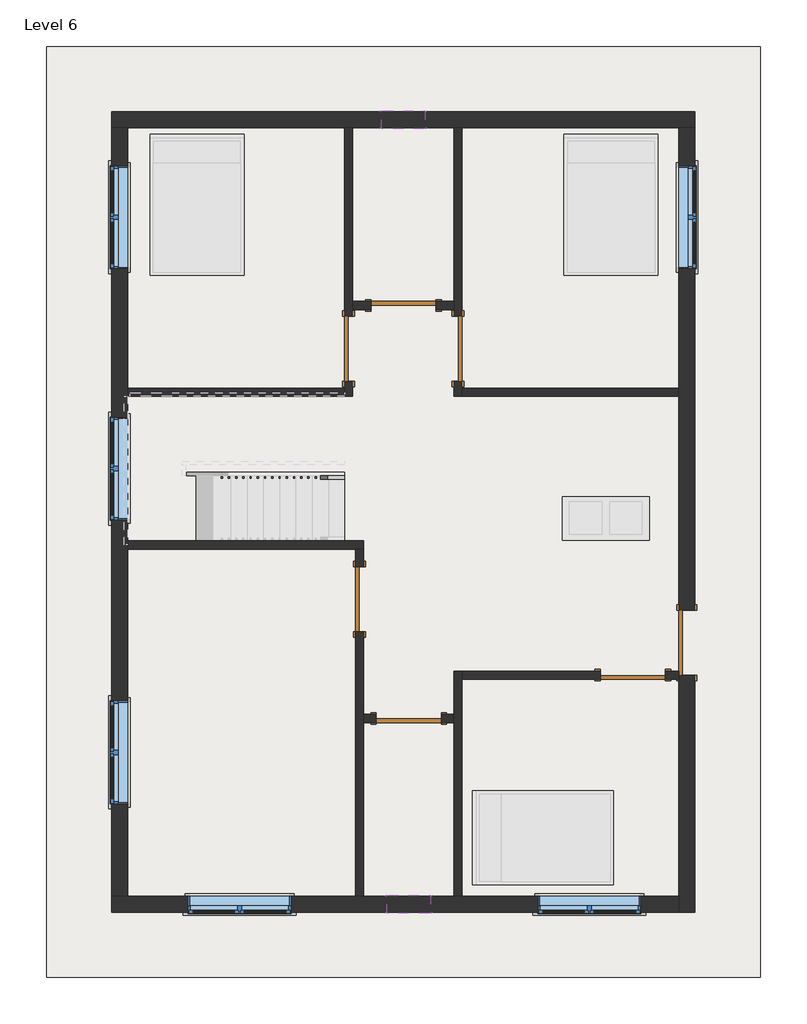
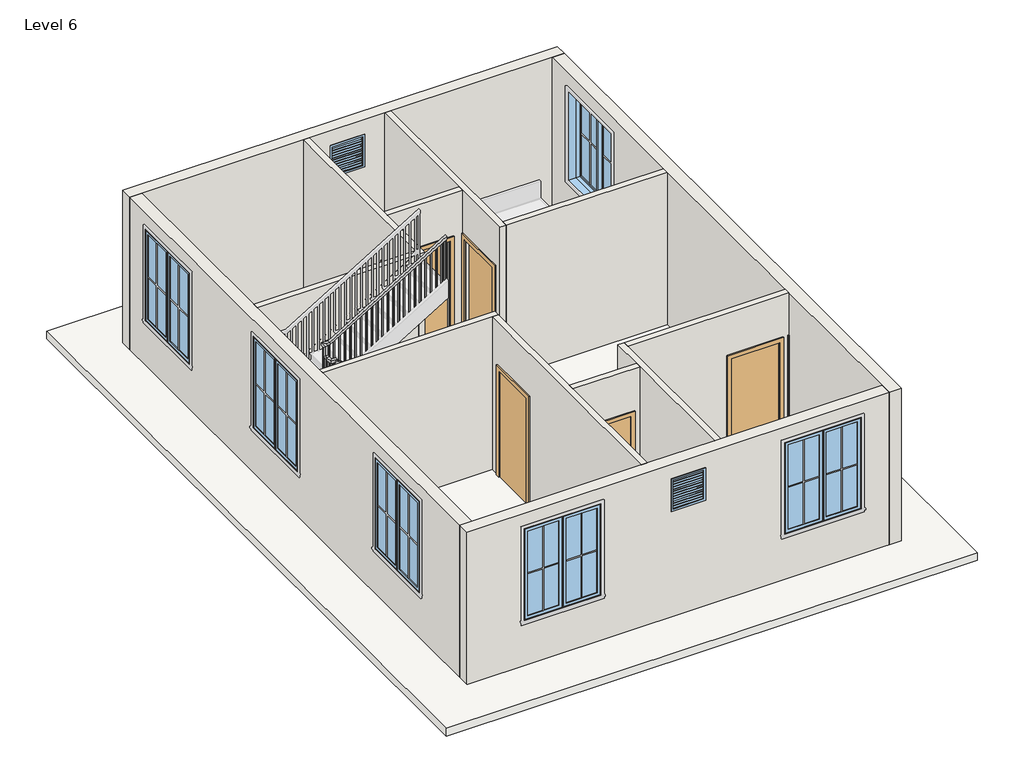
# One storey, part 1 of 2: 14 walls, 8 windows, 7 doors, 1 railing, 1 roof, 1 slab.
"""IFC4 building model written with IfcOpenShell, lengths in millimetres."""

from ifc_helpers import new_model, si_unit, frame, origin, place, context, project, spatial, polyline, outline, extrude, faceted_brep, transform, mapped, element, save
from components import door_305aa2a5, door_e5f9f3c4, door_0ca8825f, window_9ac97e1a, window_f2d8fef0

model = new_model("IFC4")

# Units and contexts
model_context = context("Model", 3, world=origin())
ifc_project = project(units=[si_unit("LENGTHUNIT", "METRE", prefix="MILLI")], contexts=[model_context])

# Site, building, storey
site = spatial("IfcSite", under=ifc_project)
building = spatial("IfcBuilding", under=site)
storey = spatial("IfcBuildingStorey", under=building, Name="Level 6", Elevation=12801.6)

# Doors
placement = place(None, origin())
door_shape = door_305aa2a5(model_context)
element("IfcDoor", 1, ObjectType="Single-Flush : 36\" x 84\"", at=placement, inside=storey, context=model_context, shape_type="MappedRepresentation", body=[
    mapped(door_shape, transform((-2023.6910855, 2116.5303617, 12801.6), x_axis=(0.0, -1.0, 0.0), y_axis=(1.0, 0.0, 0.0), z_axis=(0.0, 0.0, 1.0))),
])
element("IfcDoor", 2, ObjectType="Single-Flush : 36\" x 84\"", at=placement, inside=storey, context=model_context, shape_type="MappedRepresentation", body=[
    mapped(door_shape, transform((-1179.1410855, -3078.1725945, 12801.6), x_axis=(1.0, 0.0, 0.0), y_axis=(0.0, 1.0, 0.0), z_axis=(0.0, 0.0, 1.0))),
])
element("IfcDoor", 3, ObjectType="Single-Flush : 36\" x 84\"", at=placement, inside=storey, context=model_context, shape_type="MappedRepresentation", body=[
    mapped(door_shape, transform((1970.4589145, -2468.1696383, 12801.6), x_axis=(1.0, 0.0, 0.0), y_axis=(0.0, 1.0, 0.0), z_axis=(0.0, 0.0, 1.0))),
])
door_2_shape = door_e5f9f3c4(model_context)
element("IfcDoor", 4, ObjectType="Single-Flush : 36\" x 84\"", at=placement, inside=storey, context=model_context, shape_type="MappedRepresentation", body=[
    mapped(door_2_shape, transform((-486.9910855, 2116.5303617, 12801.6), x_axis=(0.0, -1.0, 0.0), y_axis=(1.0, 0.0, 0.0), z_axis=(0.0, 0.0, 1.0))),
])
element("IfcDoor", 5, ObjectType="Single-Flush : 36\" x 84\"", at=placement, inside=storey, context=model_context, shape_type="MappedRepresentation", body=[
    mapped(door_2_shape, transform((-1871.2910855, -1401.3696383, 12801.6), x_axis=(0.0, 1.0, 0.0), y_axis=(-1.0, 0.0, 0.0), z_axis=(0.0, 0.0, 1.0))),
])
element("IfcDoor", 6, ObjectType="Single-Flush : 36\" x 84\"", at=placement, inside=storey, context=model_context, shape_type="MappedRepresentation", body=[
    mapped(door_2_shape, transform((-1255.3410855, 2726.1303617, 12801.6), x_axis=(1.0, 0.0, 0.0), y_axis=(0.0, 1.0, 0.0), z_axis=(0.0, 0.0, 1.0))),
])
door_3_shape = door_0ca8825f(model_context)
element("IfcDoor", 7, ObjectType="Single-Flush : 36\" x 84\"", at=placement, inside=storey, context=model_context, shape_type="MappedRepresentation", body=[
    mapped(door_3_shape, transform((2732.4589145, -2010.9696383, 12801.6), x_axis=(0.0, 1.0, 0.0), y_axis=(-1.0, 0.0, 0.0), z_axis=(0.0, 0.0, 1.0))),
])

# Railing
element("IfcRailing", 8, ObjectType="Handrail - Rectangular", at=placement, inside=storey, context=model_context, shape_type="SolidModel", body=[
    faceted_brep([(-2080.8410855, 281.3803617, 13854.5454545), (-2080.8410855, 281.3803617, 13795.1439943), (-2080.8410855, 332.1803617, 13795.1439943), (-2080.8410855, 332.1803617, 13854.5454545), (-4290.6410855, 281.3803617, 15193.8181818), (-4341.4410855, 281.3803617, 15165.2046004), (-4341.4410855, 332.1803617, 15165.2046004), (-4290.6410855, 332.1803617, 15193.8181818), (-4290.6410855, 281.3803617, 15240.0), (-4341.4410855, 281.3803617, 15189.2), (-4341.4410855, 332.1803617, 15189.2), (-4290.6410855, 332.1803617, 15240.0), (-4417.6410855, 281.3803617, 15240.0), (-4417.6410855, 281.3803617, 15189.2), (-4366.8410855, 332.1803617, 15189.2), (-4366.8410855, 332.1803617, 15240.0), (-4417.6410855, 408.3803617, 15240.0), (-4417.6410855, 408.3803617, 15189.2), (-4366.8410855, 408.3803617, 15189.2), (-4366.8410855, 408.3803617, 15240.0), (-4417.6410855, 459.1803617, 15240.0), (-4417.6410855, 509.9803617, 15189.2), (-4366.8410855, 509.9803617, 15189.2), (-4366.8410855, 459.1803617, 15240.0), (-4417.6410855, 459.1803617, 15424.7272727), (-4417.6410855, 509.9803617, 15373.9272727), (-4366.8410855, 509.9803617, 15373.9272727), (-4366.8410855, 459.1803617, 15424.7272727), (-4417.6410855, 586.1803617, 15424.7272727), (-4417.6410855, 586.1803617, 15373.9272727), (-4366.8410855, 535.3803617, 15373.9272727), (-4366.8410855, 535.3803617, 15424.7272727), (-4290.6410855, 586.1803617, 15424.7272727), (-4276.4486761, 586.1803617, 15373.9272727), (-4276.4486761, 535.3803617, 15373.9272727), (-4290.6410855, 535.3803617, 15424.7272727), (-2080.8410855, 586.1803617, 16764.0), (-2080.8410855, 535.3803617, 16764.0), (-2080.8410855, 535.3803617, 16704.5985397), (-2080.8410855, 586.1803617, 16704.5985397)], [[[0, 1, 2, 3]], [[1, 0, 4, 5]], [[2, 1, 5, 6]], [[3, 2, 6, 7]], [[0, 3, 7, 4]], [[5, 4, 8, 9]], [[6, 5, 9, 10]], [[7, 6, 10, 11]], [[4, 7, 11, 8]], [[9, 8, 12, 13]], [[10, 9, 13, 14]], [[11, 10, 14, 15]], [[8, 11, 15, 12]], [[13, 12, 16, 17]], [[14, 13, 17, 18]], [[15, 14, 18, 19]], [[12, 15, 19, 16]], [[17, 16, 20, 21]], [[18, 17, 21, 22]], [[19, 18, 22, 23]], [[16, 19, 23, 20]], [[21, 20, 24, 25]], [[22, 21, 25, 26]], [[23, 22, 26, 27]], [[20, 23, 27, 24]], [[25, 24, 28, 29]], [[26, 25, 29, 30]], [[27, 26, 30, 31]], [[24, 27, 31, 28]], [[29, 28, 32, 33]], [[30, 29, 33, 34]], [[31, 30, 34, 35]], [[28, 31, 35, 32]], [[36, 37, 38, 39]], [[33, 32, 36, 39]], [[34, 33, 39, 38]], [[35, 34, 38, 37]], [[32, 35, 37, 36]]]),
    extrude(outline(polyline([(16664.1894488, -2147.5160855), (16652.6439943, -2166.5660855), (15711.0545455, -2166.5660855), (15711.0545455, -2147.5160855), (16664.1894488, -2147.5160855)])), frame((0.0, 551.2553617, 0.0), z_axis=(0.0, 1.0, 0.0), x_axis=(0.0, 0.0, 1.0)), (0.0, 0.0, 1.0), 19.05),
    extrude(outline(polyline([(16602.6136913, -2249.1160855), (16591.0682367, -2268.1660855), (15711.0545455, -2268.1660855), (15711.0545455, -2249.1160855), (16602.6136913, -2249.1160855)])), frame((0.0, 551.2553617, 0.0), z_axis=(0.0, 1.0, 0.0), x_axis=(0.0, 0.0, 1.0)), (0.0, 0.0, 1.0), 19.05),
    extrude(outline(polyline([(16541.0379337, -2350.7160855), (16529.4924791, -2369.7660855), (15572.5090909, -2369.7660855), (15572.5090909, -2350.7160855), (16541.0379337, -2350.7160855)])), frame((0.0, 551.2553617, 0.0), z_axis=(0.0, 1.0, 0.0), x_axis=(0.0, 0.0, 1.0)), (0.0, 0.0, 1.0), 19.05),
    extrude(outline(polyline([(16479.4621761, -2452.3160855), (16467.9167216, -2471.3660855), (15572.5090909, -2471.3660855), (15572.5090909, -2452.3160855), (16479.4621761, -2452.3160855)])), frame((0.0, 551.2553617, 0.0), z_axis=(0.0, 1.0, 0.0), x_axis=(0.0, 0.0, 1.0)), (0.0, 0.0, 1.0), 19.05),
    extrude(outline(polyline([(16417.8864185, -2553.9160855), (16406.340964, -2572.9660855), (15433.9636364, -2572.9660855), (15433.9636364, -2553.9160855), (16417.8864185, -2553.9160855)])), frame((0.0, 551.2553617, 0.0), z_axis=(0.0, 1.0, 0.0), x_axis=(0.0, 0.0, 1.0)), (0.0, 0.0, 1.0), 19.05),
    extrude(outline(polyline([(16356.310661, -2655.5160855), (16344.7652064, -2674.5660855), (15433.9636364, -2674.5660855), (15433.9636364, -2655.5160855), (16356.310661, -2655.5160855)])), frame((0.0, 551.2553617, 0.0), z_axis=(0.0, 1.0, 0.0), x_axis=(0.0, 0.0, 1.0)), (0.0, 0.0, 1.0), 19.05),
    extrude(outline(polyline([(16294.7349034, -2757.1160855), (16283.1894488, -2776.1660855), (15433.9636364, -2776.1660855), (15433.9636364, -2757.1160855), (16294.7349034, -2757.1160855)])), frame((0.0, 551.2553617, 0.0), z_axis=(0.0, 1.0, 0.0), x_axis=(0.0, 0.0, 1.0)), (0.0, 0.0, 1.0), 19.05),
    extrude(outline(polyline([(16233.1591458, -2858.7160855), (16221.6136913, -2877.7660855), (15295.4181818, -2877.7660855), (15295.4181818, -2858.7160855), (16233.1591458, -2858.7160855)])), frame((0.0, 551.2553617, 0.0), z_axis=(0.0, 1.0, 0.0), x_axis=(0.0, 0.0, 1.0)), (0.0, 0.0, 1.0), 19.05),
    extrude(outline(polyline([(16171.5833882, -2960.3160855), (16160.0379337, -2979.3660855), (15295.4181818, -2979.3660855), (15295.4181818, -2960.3160855), (16171.5833882, -2960.3160855)])), frame((0.0, 551.2553617, 0.0), z_axis=(0.0, 1.0, 0.0), x_axis=(0.0, 0.0, 1.0)), (0.0, 0.0, 1.0), 19.05),
    extrude(outline(polyline([(16110.0076307, -3061.9160855), (16098.4621761, -3080.9660855), (15156.8727273, -3080.9660855), (15156.8727273, -3061.9160855), (16110.0076307, -3061.9160855)])), frame((0.0, 551.2553617, 0.0), z_axis=(0.0, 1.0, 0.0), x_axis=(0.0, 0.0, 1.0)), (0.0, 0.0, 1.0), 19.05),
    extrude(outline(polyline([(16048.4318731, -3163.5160855), (16036.8864185, -3182.5660855), (15156.8727273, -3182.5660855), (15156.8727273, -3163.5160855), (16048.4318731, -3163.5160855)])), frame((0.0, 551.2553617, 0.0), z_axis=(0.0, 1.0, 0.0), x_axis=(0.0, 0.0, 1.0)), (0.0, 0.0, 1.0), 19.05),
    extrude(outline(polyline([(15986.8561155, -3265.1160855), (15975.310661, -3284.1660855), (15018.3272727, -3284.1660855), (15018.3272727, -3265.1160855), (15986.8561155, -3265.1160855)])), frame((0.0, 551.2553617, 0.0), z_axis=(0.0, 1.0, 0.0), x_axis=(0.0, 0.0, 1.0)), (0.0, 0.0, 1.0), 19.05),
    extrude(outline(polyline([(15925.2803579, -3366.7160855), (15913.7349034, -3385.7660855), (15018.3272727, -3385.7660855), (15018.3272727, -3366.7160855), (15925.2803579, -3366.7160855)])), frame((0.0, 551.2553617, 0.0), z_axis=(0.0, 1.0, 0.0), x_axis=(0.0, 0.0, 1.0)), (0.0, 0.0, 1.0), 19.05),
    extrude(outline(polyline([(15863.7046004, -3468.3160855), (15852.1591458, -3487.3660855), (14879.7818182, -3487.3660855), (14879.7818182, -3468.3160855), (15863.7046004, -3468.3160855)])), frame((0.0, 551.2553617, 0.0), z_axis=(0.0, 1.0, 0.0), x_axis=(0.0, 0.0, 1.0)), (0.0, 0.0, 1.0), 19.05),
    extrude(outline(polyline([(15802.1288428, -3569.9160855), (15790.5833882, -3588.9660855), (14879.7818182, -3588.9660855), (14879.7818182, -3569.9160855), (15802.1288428, -3569.9160855)])), frame((0.0, 551.2553617, 0.0), z_axis=(0.0, 1.0, 0.0), x_axis=(0.0, 0.0, 1.0)), (0.0, 0.0, 1.0), 19.05),
    extrude(outline(polyline([(15740.5530852, -3671.5160855), (15729.0076307, -3690.5660855), (14879.7818182, -3690.5660855), (14879.7818182, -3671.5160855), (15740.5530852, -3671.5160855)])), frame((0.0, 551.2553617, 0.0), z_axis=(0.0, 1.0, 0.0), x_axis=(0.0, 0.0, 1.0)), (0.0, 0.0, 1.0), 19.05),
    extrude(outline(polyline([(15678.9773276, -3773.1160855), (15667.4318731, -3792.1660855), (14741.2363636, -3792.1660855), (14741.2363636, -3773.1160855), (15678.9773276, -3773.1160855)])), frame((0.0, 551.2553617, 0.0), z_axis=(0.0, 1.0, 0.0), x_axis=(0.0, 0.0, 1.0)), (0.0, 0.0, 1.0), 19.05),
    extrude(outline(polyline([(15617.40157, -3874.7160855), (15605.8561155, -3893.7660855), (14741.2363636, -3893.7660855), (14741.2363636, -3874.7160855), (15617.40157, -3874.7160855)])), frame((0.0, 551.2553617, 0.0), z_axis=(0.0, 1.0, 0.0), x_axis=(0.0, 0.0, 1.0)), (0.0, 0.0, 1.0), 19.05),
    extrude(outline(polyline([(15555.8258125, -3976.3160855), (15544.2803579, -3995.3660855), (14602.6909091, -3995.3660855), (14602.6909091, -3976.3160855), (15555.8258125, -3976.3160855)])), frame((0.0, 551.2553617, 0.0), z_axis=(0.0, 1.0, 0.0), x_axis=(0.0, 0.0, 1.0)), (0.0, 0.0, 1.0), 19.05),
    extrude(outline(polyline([(15494.2500549, -4077.9160855), (15482.7046004, -4096.9660855), (14602.6909091, -4096.9660855), (14602.6909091, -4077.9160855), (15494.2500549, -4077.9160855)])), frame((0.0, 551.2553617, 0.0), z_axis=(0.0, 1.0, 0.0), x_axis=(0.0, 0.0, 1.0)), (0.0, 0.0, 1.0), 19.05),
    extrude(outline(polyline([(15432.6742973, -4179.5160855), (15421.1288428, -4198.5660855), (14464.1454545, -4198.5660855), (14464.1454545, -4179.5160855), (15432.6742973, -4179.5160855)])), frame((0.0, 551.2553617, 0.0), z_axis=(0.0, 1.0, 0.0), x_axis=(0.0, 0.0, 1.0)), (0.0, 0.0, 1.0), 19.05),
    extrude(outline(polyline([(15371.0985397, -4281.1160855), (15359.5530852, -4300.1660855), (14464.1454545, -4300.1660855), (14464.1454545, -4281.1160855), (15371.0985397, -4281.1160855)])), frame((0.0, 551.2553617, 0.0), z_axis=(0.0, 1.0, 0.0), x_axis=(0.0, 0.0, 1.0)), (0.0, 0.0, 1.0), 19.05),
    extrude(outline(polyline([(-4382.7160855, 500.4553617), (-4401.7660855, 500.4553617), (-4401.7660855, 519.5053617), (-4382.7160855, 519.5053617), (-4382.7160855, 500.4553617)])), frame((0.0, 0.0, 14325.6), z_axis=(0.0, 0.0, 1.0), x_axis=(1.0, 0.0, 0.0)), (0.0, 0.0, 1.0), 1048.3272727),
    extrude(outline(polyline([(-4382.7160855, 398.8553617), (-4401.7660855, 398.8553617), (-4401.7660855, 417.9053617), (-4382.7160855, 417.9053617), (-4382.7160855, 398.8553617)])), frame((0.0, 0.0, 14325.6), z_axis=(0.0, 0.0, 1.0), x_axis=(1.0, 0.0, 0.0)), (0.0, 0.0, 1.0), 863.6),
    extrude(outline(polyline([(-4306.5160855, 316.3053617), (-4306.5160855, 297.2553617), (-4325.5660855, 297.2553617), (-4325.5660855, 316.3053617), (-4306.5160855, 316.3053617)])), frame((0.0, 0.0, 14187.0545455), z_axis=(0.0, 0.0, 1.0), x_axis=(1.0, 0.0, 0.0)), (0.0, 0.0, 1.0), 1002.1454545),
    extrude(outline(polyline([(15082.4621761, -4204.9160855), (15094.0076307, -4223.9660855), (14187.0545455, -4223.9660855), (14187.0545455, -4204.9160855), (15082.4621761, -4204.9160855)])), frame((0.0, 297.2553617, 0.0), z_axis=(0.0, 1.0, 0.0), x_axis=(0.0, 0.0, 1.0)), (0.0, 0.0, 1.0), 19.05),
    extrude(outline(polyline([(15020.8864185, -4103.3160855), (15032.4318731, -4122.3660855), (14048.5090909, -4122.3660855), (14048.5090909, -4103.3160855), (15020.8864185, -4103.3160855)])), frame((0.0, 297.2553617, 0.0), z_axis=(0.0, 1.0, 0.0), x_axis=(0.0, 0.0, 1.0)), (0.0, 0.0, 1.0), 19.05),
    extrude(outline(polyline([(14959.310661, -4001.7160855), (14970.8561155, -4020.7660855), (14048.5090909, -4020.7660855), (14048.5090909, -4001.7160855), (14959.310661, -4001.7160855)])), frame((0.0, 297.2553617, 0.0), z_axis=(0.0, 1.0, 0.0), x_axis=(0.0, 0.0, 1.0)), (0.0, 0.0, 1.0), 19.05),
    extrude(outline(polyline([(14897.7349034, -3900.1160855), (14909.2803579, -3919.1660855), (14048.5090909, -3919.1660855), (14048.5090909, -3900.1160855), (14897.7349034, -3900.1160855)])), frame((0.0, 297.2553617, 0.0), z_axis=(0.0, 1.0, 0.0), x_axis=(0.0, 0.0, 1.0)), (0.0, 0.0, 1.0), 19.05),
    extrude(outline(polyline([(14836.1591458, -3798.5160855), (14847.7046004, -3817.5660855), (13909.9636364, -3817.5660855), (13909.9636364, -3798.5160855), (14836.1591458, -3798.5160855)])), frame((0.0, 297.2553617, 0.0), z_axis=(0.0, 1.0, 0.0), x_axis=(0.0, 0.0, 1.0)), (0.0, 0.0, 1.0), 19.05),
    extrude(outline(polyline([(14774.5833882, -3696.9160855), (14786.1288428, -3715.9660855), (13909.9636364, -3715.9660855), (13909.9636364, -3696.9160855), (14774.5833882, -3696.9160855)])), frame((0.0, 297.2553617, 0.0), z_axis=(0.0, 1.0, 0.0), x_axis=(0.0, 0.0, 1.0)), (0.0, 0.0, 1.0), 19.05),
    extrude(outline(polyline([(14713.0076307, -3595.3160855), (14724.5530852, -3614.3660855), (13771.4181818, -3614.3660855), (13771.4181818, -3595.3160855), (14713.0076307, -3595.3160855)])), frame((0.0, 297.2553617, 0.0), z_axis=(0.0, 1.0, 0.0), x_axis=(0.0, 0.0, 1.0)), (0.0, 0.0, 1.0), 19.05),
    extrude(outline(polyline([(14651.4318731, -3493.7160855), (14662.9773276, -3512.7660855), (13771.4181818, -3512.7660855), (13771.4181818, -3493.7160855), (14651.4318731, -3493.7160855)])), frame((0.0, 297.2553617, 0.0), z_axis=(0.0, 1.0, 0.0), x_axis=(0.0, 0.0, 1.0)), (0.0, 0.0, 1.0), 19.05),
    extrude(outline(polyline([(14589.8561155, -3392.1160855), (14601.40157, -3411.1660855), (13632.8727273, -3411.1660855), (13632.8727273, -3392.1160855), (14589.8561155, -3392.1160855)])), frame((0.0, 297.2553617, 0.0), z_axis=(0.0, 1.0, 0.0), x_axis=(0.0, 0.0, 1.0)), (0.0, 0.0, 1.0), 19.05),
    extrude(outline(polyline([(14528.2803579, -3290.5160855), (14539.8258125, -3309.5660855), (13632.8727273, -3309.5660855), (13632.8727273, -3290.5160855), (14528.2803579, -3290.5160855)])), frame((0.0, 297.2553617, 0.0), z_axis=(0.0, 1.0, 0.0), x_axis=(0.0, 0.0, 1.0)), (0.0, 0.0, 1.0), 19.05),
    extrude(outline(polyline([(14466.7046004, -3188.9160855), (14478.2500549, -3207.9660855), (13494.3272727, -3207.9660855), (13494.3272727, -3188.9160855), (14466.7046004, -3188.9160855)])), frame((0.0, 297.2553617, 0.0), z_axis=(0.0, 1.0, 0.0), x_axis=(0.0, 0.0, 1.0)), (0.0, 0.0, 1.0), 19.05),
    extrude(outline(polyline([(14405.1288428, -3087.3160855), (14416.6742973, -3106.3660855), (13494.3272727, -3106.3660855), (13494.3272727, -3087.3160855), (14405.1288428, -3087.3160855)])), frame((0.0, 297.2553617, 0.0), z_axis=(0.0, 1.0, 0.0), x_axis=(0.0, 0.0, 1.0)), (0.0, 0.0, 1.0), 19.05),
    extrude(outline(polyline([(14343.5530852, -2985.7160855), (14355.0985397, -3004.7660855), (13494.3272727, -3004.7660855), (13494.3272727, -2985.7160855), (14343.5530852, -2985.7160855)])), frame((0.0, 297.2553617, 0.0), z_axis=(0.0, 1.0, 0.0), x_axis=(0.0, 0.0, 1.0)), (0.0, 0.0, 1.0), 19.05),
    extrude(outline(polyline([(14281.9773276, -2884.1160855), (14293.5227822, -2903.1660855), (13355.7818182, -2903.1660855), (13355.7818182, -2884.1160855), (14281.9773276, -2884.1160855)])), frame((0.0, 297.2553617, 0.0), z_axis=(0.0, 1.0, 0.0), x_axis=(0.0, 0.0, 1.0)), (0.0, 0.0, 1.0), 19.05),
    extrude(outline(polyline([(14220.40157, -2782.5160855), (14231.9470246, -2801.5660855), (13355.7818182, -2801.5660855), (13355.7818182, -2782.5160855), (14220.40157, -2782.5160855)])), frame((0.0, 297.2553617, 0.0), z_axis=(0.0, 1.0, 0.0), x_axis=(0.0, 0.0, 1.0)), (0.0, 0.0, 1.0), 19.05),
    extrude(outline(polyline([(14158.8258125, -2680.9160855), (14170.371267, -2699.9660855), (13217.2363636, -2699.9660855), (13217.2363636, -2680.9160855), (14158.8258125, -2680.9160855)])), frame((0.0, 297.2553617, 0.0), z_axis=(0.0, 1.0, 0.0), x_axis=(0.0, 0.0, 1.0)), (0.0, 0.0, 1.0), 19.05),
    extrude(outline(polyline([(14097.2500549, -2579.3160855), (14108.7955094, -2598.3660855), (13217.2363636, -2598.3660855), (13217.2363636, -2579.3160855), (14097.2500549, -2579.3160855)])), frame((0.0, 297.2553617, 0.0), z_axis=(0.0, 1.0, 0.0), x_axis=(0.0, 0.0, 1.0)), (0.0, 0.0, 1.0), 19.05),
    extrude(outline(polyline([(14035.6742973, -2477.7160855), (14047.2197519, -2496.7660855), (13078.6909091, -2496.7660855), (13078.6909091, -2477.7160855), (14035.6742973, -2477.7160855)])), frame((0.0, 297.2553617, 0.0), z_axis=(0.0, 1.0, 0.0), x_axis=(0.0, 0.0, 1.0)), (0.0, 0.0, 1.0), 19.05),
    extrude(outline(polyline([(13974.0985397, -2376.1160855), (13985.6439943, -2395.1660855), (13078.6909091, -2395.1660855), (13078.6909091, -2376.1160855), (13974.0985397, -2376.1160855)])), frame((0.0, 297.2553617, 0.0), z_axis=(0.0, 1.0, 0.0), x_axis=(0.0, 0.0, 1.0)), (0.0, 0.0, 1.0), 19.05),
    extrude(outline(polyline([(13912.5227822, -2274.5160855), (13924.0682367, -2293.5660855), (12940.1454545, -2293.5660855), (12940.1454545, -2274.5160855), (13912.5227822, -2274.5160855)])), frame((0.0, 297.2553617, 0.0), z_axis=(0.0, 1.0, 0.0), x_axis=(0.0, 0.0, 1.0)), (0.0, 0.0, 1.0), 19.05),
    extrude(outline(polyline([(13850.9470246, -2172.9160855), (13862.4924791, -2191.9660855), (12940.1454545, -2191.9660855), (12940.1454545, -2172.9160855), (13850.9470246, -2172.9160855)])), frame((0.0, 297.2553617, 0.0), z_axis=(0.0, 1.0, 0.0), x_axis=(0.0, 0.0, 1.0)), (0.0, 0.0, 1.0), 19.05),
    extrude(outline(polyline([(-4382.7160855, 551.2553617), (-4401.7660855, 551.2553617), (-4401.7660855, 570.3053617), (-4382.7160855, 570.3053617), (-4382.7160855, 551.2553617)])), frame((0.0, 0.0, 14325.6), z_axis=(0.0, 0.0, 1.0), x_axis=(1.0, 0.0, 0.0)), (0.0, 0.0, 1.0), 1048.3272727),
    extrude(outline(polyline([(-4382.7160855, 316.3053617), (-4382.7160855, 297.2553617), (-4401.7660855, 297.2553617), (-4401.7660855, 316.3053617), (-4382.7160855, 316.3053617)])), frame((0.0, 0.0, 14325.6), z_axis=(0.0, 0.0, 1.0), x_axis=(1.0, 0.0, 0.0)), (0.0, 0.0, 1.0), 863.6),
    extrude(outline(polyline([(16704.5985397, -2080.8410855), (16693.0530852, -2099.8910855), (15711.0545455, -2099.8910855), (15711.0545455, -2080.8410855), (16704.5985397, -2080.8410855)])), frame((0.0, 551.2553617, 0.0), z_axis=(0.0, 1.0, 0.0), x_axis=(0.0, 0.0, 1.0)), (0.0, 0.0, 1.0), 19.05),
    extrude(outline(polyline([(13795.1439943, -2080.8410855), (13806.6894488, -2099.8910855), (12940.1454545, -2099.8910855), (12940.1454545, -2080.8410855), (13795.1439943, -2080.8410855)])), frame((0.0, 297.2553617, 0.0), z_axis=(0.0, 1.0, 0.0), x_axis=(0.0, 0.0, 1.0)), (0.0, 0.0, 1.0), 19.05),
])

# Roof
element("IfcRoof", 9, ObjectType="ROOF 6\"", at=placement, inside=storey, context=model_context, shape_type="SweptSolid", body=[
    extrude(outline(polyline([(-6271.8410855, 6364.6803617), (3761.1589145, 6364.6803617), (3761.1589145, -6716.3196383), (-6271.8410855, -6716.3196383), (-6271.8410855, 6364.6803617)])), frame((0.0, 0.0, 12649.2), z_axis=(0.0, 0.0, 1.0), x_axis=(1.0, 0.0, 0.0)), (0.0, 0.0, 1.0), 152.4),
])

# Slab
element("IfcSlab", 10, ObjectType="FLOOR 6\"", at=placement, inside=storey, context=model_context, shape_type="SweptSolid", body=[
    extrude(outline(polyline([(2846.7589145, 5450.2803617), (2846.7589145, -5801.9196383), (-5357.4410855, -5801.9196383), (-5357.4410855, 5450.2803617), (2846.7589145, 5450.2803617)])), frame((0.0, 0.0, 12649.2), z_axis=(0.0, 0.0, 1.0), x_axis=(1.0, 0.0, 0.0)), (0.0, 0.0, 1.0), 152.4),
])

# Walls
element("IfcWall", 11, ObjectType="WALL 4.5\"", at=placement, inside=storey, context=model_context, shape_type="Brep", body=[
    faceted_brep([(-2080.8410855, 1659.3303617, 14935.2), (-2080.8410855, 1659.3303617, 12801.6), (-2080.8410855, 1564.0803617, 12801.6), (-2080.8410855, 1449.7803617, 12801.6), (-2080.8410855, 1449.7803617, 15849.6), (-2080.8410855, 1564.0803617, 15849.6), (-2080.8410855, 5221.6803617, 15849.6), (-2080.8410855, 5221.6803617, 12801.6), (-2080.8410855, 2573.7303617, 12801.6), (-2080.8410855, 2573.7303617, 14935.2), (-1966.5410855, 1449.7803617, 12801.6), (-1966.5410855, 1659.3303617, 12801.6), (-1966.5410855, 1659.3303617, 14935.2), (-1966.5410855, 2573.7303617, 14935.2), (-1966.5410855, 2573.7303617, 12801.6), (-1966.5410855, 2668.9803617, 12801.6), (-1966.5410855, 2783.2803617, 12801.6), (-1966.5410855, 5221.6803617, 12801.6), (-1966.5410855, 5221.6803617, 15849.6), (-1966.5410855, 2783.2803617, 15849.6), (-1966.5410855, 2668.9803617, 15849.6), (-1966.5410855, 1449.7803617, 15849.6)], [[[0, 1, 2, 3, 4, 5, 6, 7, 8, 9]], [[10, 11, 12, 13, 14, 15, 16, 17, 18, 19, 20, 21]], [[8, 7, 17, 16, 15, 14]], [[3, 2, 1, 11, 10]], [[7, 6, 18, 17]], [[4, 3, 10, 21]], [[12, 11, 1, 0]], [[13, 12, 0, 9]], [[14, 13, 9, 8]], [[6, 5, 4, 21, 20, 19, 18]]]),
])
element("IfcWall", 12, ObjectType="WALL 4.5\"", at=placement, inside=storey, context=model_context, shape_type="SweptSolid", body=[
    extrude(outline(polyline([(-5128.8410855, 1564.0803617), (-2080.8410855, 1564.0803617), (-2080.8410855, 1449.7803617), (-5128.8410855, 1449.7803617), (-5128.8410855, 1564.0803617)])), frame((0.0, 0.0, 12801.6), z_axis=(0.0, 0.0, 1.0), x_axis=(1.0, 0.0, 0.0)), (0.0, 0.0, 1.0), 3048.0),
])
element("IfcWall", 13, ObjectType="WALL 4.5\"", at=placement, inside=storey, context=model_context, shape_type="Brep", body=[
    faceted_brep([(-544.1410855, 1659.3303617, 14935.2), (-544.1410855, 1659.3303617, 12801.6), (-544.1410855, 1449.7803617, 12801.6), (-544.1410855, 1449.7803617, 15849.6), (-544.1410855, 2668.9803617, 15849.6), (-544.1410855, 2783.2803617, 15849.6), (-544.1410855, 5221.6803617, 15849.6), (-544.1410855, 5221.6803617, 12801.6), (-544.1410855, 2783.2803617, 12801.6), (-544.1410855, 2668.9803617, 12801.6), (-544.1410855, 2573.7303617, 12801.6), (-544.1410855, 2573.7303617, 14935.2), (-429.8410855, 1449.7803617, 12801.6), (-429.8410855, 1564.0803617, 12801.6), (-429.8410855, 1659.3303617, 12801.6), (-429.8410855, 1659.3303617, 14935.2), (-429.8410855, 2573.7303617, 14935.2), (-429.8410855, 2573.7303617, 12801.6), (-429.8410855, 5221.6803617, 12801.6), (-429.8410855, 5221.6803617, 15849.6), (-429.8410855, 1564.0803617, 15849.6), (-429.8410855, 1449.7803617, 15849.6)], [[[0, 1, 2, 3, 4, 5, 6, 7, 8, 9, 10, 11]], [[12, 13, 14, 15, 16, 17, 18, 19, 20, 21]], [[2, 1, 14, 13, 12]], [[10, 9, 8, 7, 18, 17]], [[7, 6, 19, 18]], [[3, 2, 12, 21]], [[15, 14, 1, 0]], [[16, 15, 0, 11]], [[17, 16, 11, 10]], [[6, 5, 4, 3, 21, 20, 19]]]),
])
element("IfcWall", 14, ObjectType="WALL 4.5\"", at=placement, inside=storey, context=model_context, shape_type="SweptSolid", body=[
    extrude(outline(polyline([(2618.1589145, 1449.7803617), (-429.8410855, 1449.7803617), (-429.8410855, 1564.0803617), (2618.1589145, 1564.0803617), (2618.1589145, 1449.7803617)])), frame((0.0, 0.0, 12801.6), z_axis=(0.0, 0.0, 1.0), x_axis=(1.0, 0.0, 0.0)), (0.0, 0.0, 1.0), 3048.0),
])
element("IfcWall", 15, ObjectType="WALL 4.5\"", at=placement, inside=storey, context=model_context, shape_type="Brep", body=[
    faceted_brep([(-5128.8410855, -696.5196383, 12801.6), (-1928.4410855, -696.5196383, 12801.6), (-1814.1410855, -696.5196383, 12801.6), (-1814.1410855, -696.5196383, 15849.6), (-1928.4410855, -696.5196383, 15849.6), (-5128.8410855, -696.5196383, 15849.6), (-5128.8410855, -582.2196383, 12801.6), (-5128.8410855, -582.2196383, 15849.6), (-1814.1410855, -582.2196383, 15849.6), (-1814.1410855, -582.2196383, 12801.6)], [[[0, 1, 2, 3, 4, 5]], [[6, 7, 8, 9]], [[2, 1, 0, 6, 9]], [[0, 5, 7, 6]], [[3, 2, 9, 8]], [[5, 4, 3, 8, 7]]]),
])
element("IfcWall", 16, ObjectType="WALL 4.5\"", at=placement, inside=storey, context=model_context, shape_type="Brep", body=[
    faceted_brep([(-1814.1410855, -944.1696383, 14935.2), (-1814.1410855, -944.1696383, 12801.6), (-1814.1410855, -696.5196383, 12801.6), (-1814.1410855, -696.5196383, 15849.6), (-1814.1410855, -3021.0225945, 15849.6), (-1814.1410855, -3135.3225945, 15849.6), (-1814.1410855, -5573.3196383, 15849.6), (-1814.1410855, -5573.3196383, 12801.6), (-1814.1410855, -3135.3225945, 12801.6), (-1814.1410855, -3021.0225945, 12801.6), (-1814.1410855, -1858.5696383, 12801.6), (-1814.1410855, -1858.5696383, 14935.2), (-1928.4410855, -696.5196383, 12801.6), (-1928.4410855, -944.1696383, 12801.6), (-1928.4410855, -944.1696383, 14935.2), (-1928.4410855, -1858.5696383, 14935.2), (-1928.4410855, -1858.5696383, 12801.6), (-1928.4410855, -5573.3196383, 12801.6), (-1928.4410855, -5573.3196383, 15849.6), (-1928.4410855, -696.5196383, 15849.6)], [[[0, 1, 2, 3, 4, 5, 6, 7, 8, 9, 10, 11]], [[12, 13, 14, 15, 16, 17, 18, 19]], [[2, 1, 13, 12]], [[10, 9, 8, 7, 17, 16]], [[3, 2, 12, 19]], [[7, 6, 18, 17]], [[14, 13, 1, 0]], [[15, 14, 0, 11]], [[16, 15, 11, 10]], [[6, 5, 4, 3, 19, 18]]]),
])
element("IfcWall", 17, ObjectType="WALL 4.5\"", at=placement, inside=storey, context=model_context, shape_type="SweptSolid", body=[
    extrude(outline(polyline([(14935.2, -721.9410855), (12801.6, -721.9410855), (12801.6, -544.1410855), (15849.6, -544.1410855), (15849.6, -1814.1410855), (12801.6, -1814.1410855), (12801.6, -1636.3410855), (14935.2, -1636.3410855), (14935.2, -721.9410855)])), frame((0.0, -3135.3225945, 0.0), z_axis=(0.0, 1.0, 0.0), x_axis=(0.0, 0.0, 1.0)), (0.0, 0.0, 1.0), 114.3),
])
element("IfcWall", 18, ObjectType="WALL 4.5\"", at=placement, inside=storey, context=model_context, shape_type="Brep", body=[
    faceted_brep([(-544.1410855, -2411.0196383, 12801.6), (-544.1410855, -3021.0225945, 12801.6), (-544.1410855, -3135.3225945, 12801.6), (-544.1410855, -5573.3196383, 12801.6), (-544.1410855, -5573.3196383, 15849.6), (-544.1410855, -3135.3225945, 15849.6), (-544.1410855, -3021.0225945, 15849.6), (-544.1410855, -2411.0196383, 15849.6), (-429.8410855, -2411.0196383, 12801.6), (-429.8410855, -2411.0196383, 15849.6), (-429.8410855, -2525.3196383, 15849.6), (-429.8410855, -5573.3196383, 15849.6), (-429.8410855, -5573.3196383, 12801.6), (-429.8410855, -2525.3196383, 12801.6)], [[[0, 1, 2, 3, 4, 5, 6, 7]], [[8, 9, 10, 11, 12, 13]], [[3, 2, 1, 0, 8, 13, 12]], [[4, 3, 12, 11]], [[0, 7, 9, 8]], [[7, 6, 5, 4, 11, 10, 9]]]),
])
element("IfcWall", 19, ObjectType="WALL 4.5\"", at=placement, inside=storey, context=model_context, shape_type="Brep", body=[
    faceted_brep([(2427.6589145, -2525.3196383, 14935.2), (2427.6589145, -2525.3196383, 12801.6), (2618.1589145, -2525.3196383, 12801.6), (2618.1589145, -2525.3196383, 15849.6), (-429.8410855, -2525.3196383, 15849.6), (-429.8410855, -2525.3196383, 12801.6), (1513.2589145, -2525.3196383, 12801.6), (1513.2589145, -2525.3196383, 14935.2), (2618.1589145, -2411.0196383, 12801.6), (2427.6589145, -2411.0196383, 12801.6), (2427.6589145, -2411.0196383, 14935.2), (1513.2589145, -2411.0196383, 14935.2), (1513.2589145, -2411.0196383, 12801.6), (-429.8410855, -2411.0196383, 12801.6), (-429.8410855, -2411.0196383, 15849.6), (2618.1589145, -2411.0196383, 15849.6), (2618.1589145, -2468.1696383, 12801.6)], [[[0, 1, 2, 3, 4, 5, 6, 7]], [[8, 9, 10, 11, 12, 13, 14, 15]], [[6, 5, 13, 12]], [[2, 1, 9, 8, 16]], [[5, 4, 14, 13]], [[3, 2, 16, 8, 15]], [[10, 9, 1, 0]], [[11, 10, 0, 7]], [[12, 11, 7, 6]], [[4, 3, 15, 14]]]),
])
element("IfcWall", 20, ObjectType="WALL 4.5\"", at=placement, inside=storey, context=model_context, shape_type="SweptSolid", body=[
    extrude(outline(polyline([(14935.2, -798.1410855), (12801.6, -798.1410855), (12801.6, -544.1410855), (15849.6, -544.1410855), (15849.6, -1966.5410855), (12801.6, -1966.5410855), (12801.6, -1712.5410855), (14935.2, -1712.5410855), (14935.2, -798.1410855)])), frame((0.0, 2668.9803617, 0.0), z_axis=(0.0, 1.0, 0.0), x_axis=(0.0, 0.0, 1.0)), (0.0, 0.0, 1.0), 114.3),
])
element("IfcWall", 21, ObjectType="WALL 9\"", at=placement, inside=storey, context=model_context, shape_type="Brep", body=[
    faceted_brep([(-5357.4410855, 5221.6803617, 12801.6), (-5128.8410855, 5221.6803617, 12801.6), (-2080.8410855, 5221.6803617, 12801.6), (-1966.5410855, 5221.6803617, 12801.6), (-544.1410855, 5221.6803617, 12801.6), (-429.8410855, 5221.6803617, 12801.6), (2618.1589145, 5221.6803617, 12801.6), (2846.7589145, 5221.6803617, 12801.6), (2846.7589145, 5221.6803617, 15849.6), (2618.1589145, 5221.6803617, 15849.6), (-429.8410855, 5221.6803617, 15849.6), (-544.1410855, 5221.6803617, 15849.6), (-1966.5410855, 5221.6803617, 15849.6), (-2080.8410855, 5221.6803617, 15849.6), (-5128.8410855, 5221.6803617, 15849.6), (-5357.4410855, 5221.6803617, 15849.6), (-950.5410855, 5221.6803617, 15544.8), (-950.5410855, 5221.6803617, 14935.2), (-1560.1410855, 5221.6803617, 14935.2), (-1560.1410855, 5221.6803617, 15544.8), (-5357.4410855, 5450.2803617, 12801.6), (-5357.4410855, 5450.2803617, 15849.6), (2846.7589145, 5450.2803617, 15849.6), (2846.7589145, 5450.2803617, 12801.6), (-950.5410855, 5450.2803617, 15544.8), (-1560.1410855, 5450.2803617, 15544.8), (-1560.1410855, 5450.2803617, 14935.2), (-950.5410855, 5450.2803617, 14935.2)], [[[0, 1, 2, 3, 4, 5, 6, 7, 8, 9, 10, 11, 12, 13, 14, 15], [16, 17, 18, 19]], [[20, 21, 22, 23], [24, 25, 26, 27]], [[7, 6, 5, 4, 3, 2, 1, 0, 20, 23]], [[8, 7, 23, 22]], [[0, 15, 21, 20]], [[17, 16, 24, 27]], [[18, 17, 27, 26]], [[19, 18, 26, 25]], [[16, 19, 25, 24]], [[15, 14, 13, 12, 11, 10, 9, 8, 22, 21]]]),
])
element("IfcWall", 22, ObjectType="WALL 9\"", at=placement, inside=storey, context=model_context, shape_type="Brep", body=[
    faceted_brep([(2618.1589145, 5221.6803617, 12801.6), (2618.1589145, 1564.0803617, 12801.6), (2618.1589145, 1449.7803617, 12801.6), (2618.1589145, -1553.7696383, 12801.6), (2618.1589145, -1553.7696383, 14935.2), (2618.1589145, -2468.1696383, 14935.2), (2618.1589145, -2468.1696383, 12801.6), (2618.1589145, -2525.3196383, 12801.6), (2618.1589145, -5573.3196383, 12801.6), (2618.1589145, -5801.9196383, 12801.6), (2618.1589145, -5801.9196383, 15849.6), (2618.1589145, -5573.3196383, 15849.6), (2618.1589145, -2525.3196383, 15849.6), (2618.1589145, -2411.0196383, 15849.6), (2618.1589145, 1449.7803617, 15849.6), (2618.1589145, 1564.0803617, 15849.6), (2618.1589145, 5221.6803617, 15849.6), (2618.1589145, 3240.4803617, 15544.8), (2618.1589145, 3240.4803617, 13716.0), (2618.1589145, 4688.2803617, 13716.0), (2618.1589145, 4688.2803617, 15544.8), (2846.7589145, -1553.7696383, 14935.2), (2846.7589145, -1553.7696383, 12801.6), (2846.7589145, 5221.6803617, 12801.6), (2846.7589145, 5221.6803617, 15849.6), (2846.7589145, -5801.9196383, 15849.6), (2846.7589145, -5801.9196383, 12801.6), (2846.7589145, -2468.1696383, 12801.6), (2846.7589145, -2468.1696383, 14935.2), (2846.7589145, 3240.4803617, 15544.8), (2846.7589145, 4688.2803617, 15544.8), (2846.7589145, 4688.2803617, 13716.0), (2846.7589145, 3240.4803617, 13716.0)], [[[0, 1, 2, 3, 4, 5, 6, 7, 8, 9, 10, 11, 12, 13, 14, 15, 16], [17, 18, 19, 20]], [[21, 22, 23, 24, 25, 26, 27, 28], [29, 30, 31, 32]], [[27, 26, 9, 8, 7, 6]], [[23, 22, 3, 2, 1, 0]], [[0, 16, 24, 23]], [[10, 9, 26, 25]], [[18, 17, 29, 32]], [[19, 18, 32, 31]], [[20, 19, 31, 30]], [[17, 20, 30, 29]], [[4, 3, 22, 21]], [[5, 4, 21, 28]], [[6, 5, 28, 27]], [[16, 15, 14, 13, 12, 11, 10, 25, 24]]]),
])
element("IfcWall", 23, ObjectType="WALL 9\"", at=placement, inside=storey, context=model_context, shape_type="Brep", body=[
    faceted_brep([(2618.1589145, -5573.3196383, 12801.6), (-429.8410855, -5573.3196383, 12801.6), (-544.1410855, -5573.3196383, 12801.6), (-1814.1410855, -5573.3196383, 12801.6), (-1928.4410855, -5573.3196383, 12801.6), (-5128.8410855, -5573.3196383, 12801.6), (-5357.4410855, -5573.3196383, 12801.6), (-5357.4410855, -5573.3196383, 15849.6), (-5128.8410855, -5573.3196383, 15849.6), (-1928.4410855, -5573.3196383, 15849.6), (-1814.1410855, -5573.3196383, 15849.6), (-544.1410855, -5573.3196383, 15849.6), (-429.8410855, -5573.3196383, 15849.6), (2618.1589145, -5573.3196383, 15849.6), (-4281.1160855, -5573.3196383, 15544.8), (-4281.1160855, -5573.3196383, 13716.0), (-2833.3160855, -5573.3196383, 13716.0), (-2833.3160855, -5573.3196383, 15544.8), (636.9589145, -5573.3196383, 15544.8), (636.9589145, -5573.3196383, 13716.0), (2084.7589145, -5573.3196383, 13716.0), (2084.7589145, -5573.3196383, 15544.8), (-874.3410855, -5573.3196383, 15544.8), (-1483.9410855, -5573.3196383, 15544.8), (-1483.9410855, -5573.3196383, 14935.2), (-874.3410855, -5573.3196383, 14935.2), (2618.1589145, -5801.9196383, 12801.6), (2618.1589145, -5801.9196383, 15849.6), (-5357.4410855, -5801.9196383, 15849.6), (-5357.4410855, -5801.9196383, 12801.6), (-4281.1160855, -5801.9196383, 15544.8), (-2833.3160855, -5801.9196383, 15544.8), (-2833.3160855, -5801.9196383, 13716.0), (-4281.1160855, -5801.9196383, 13716.0), (636.9589145, -5801.9196383, 15544.8), (2084.7589145, -5801.9196383, 15544.8), (2084.7589145, -5801.9196383, 13716.0), (636.9589145, -5801.9196383, 13716.0), (-874.3410855, -5801.9196383, 15544.8), (-874.3410855, -5801.9196383, 14935.2), (-1483.9410855, -5801.9196383, 14935.2), (-1483.9410855, -5801.9196383, 15544.8)], [[[0, 1, 2, 3, 4, 5, 6, 7, 8, 9, 10, 11, 12, 13], [14, 15, 16, 17], [18, 19, 20, 21], [22, 23, 24, 25]], [[26, 27, 28, 29], [30, 31, 32, 33], [34, 35, 36, 37], [38, 39, 40, 41]], [[6, 5, 4, 3, 2, 1, 0, 26, 29]], [[0, 13, 27, 26]], [[7, 6, 29, 28]], [[15, 14, 30, 33]], [[16, 15, 33, 32]], [[17, 16, 32, 31]], [[14, 17, 31, 30]], [[19, 18, 34, 37]], [[20, 19, 37, 36]], [[21, 20, 36, 35]], [[18, 21, 35, 34]], [[39, 38, 22, 25]], [[40, 39, 25, 24]], [[41, 40, 24, 23]], [[38, 41, 23, 22]], [[13, 12, 11, 10, 9, 8, 7, 28, 27]]]),
])
element("IfcWall", 24, ObjectType="WALL 9\"", at=placement, inside=storey, context=model_context, shape_type="Brep", body=[
    faceted_brep([(-5128.8410855, -5573.3196383, 12801.6), (-5128.8410855, -696.5196383, 12801.6), (-5128.8410855, -582.2196383, 12801.6), (-5128.8410855, 1449.7803617, 12801.6), (-5128.8410855, 1564.0803617, 12801.6), (-5128.8410855, 5221.6803617, 12801.6), (-5128.8410855, 5221.6803617, 15849.6), (-5128.8410855, 1564.0803617, 15849.6), (-5128.8410855, 1449.7803617, 15849.6), (-5128.8410855, -582.2196383, 15849.6), (-5128.8410855, -696.5196383, 15849.6), (-5128.8410855, -5573.3196383, 15849.6), (-5128.8410855, -2830.1196383, 15544.8), (-5128.8410855, -2830.1196383, 13716.0), (-5128.8410855, -4277.9196383, 13716.0), (-5128.8410855, -4277.9196383, 15544.8), (-5128.8410855, 4688.2803617, 15544.8), (-5128.8410855, 4688.2803617, 13716.0), (-5128.8410855, 3240.4803617, 13716.0), (-5128.8410855, 3240.4803617, 15544.8), (-5128.8410855, 1157.6803617, 15544.8), (-5128.8410855, 1157.6803617, 13716.0), (-5128.8410855, -290.1196383, 13716.0), (-5128.8410855, -290.1196383, 15544.8), (-5357.4410855, -5573.3196383, 12801.6), (-5357.4410855, -5573.3196383, 15849.6), (-5357.4410855, 5221.6803617, 15849.6), (-5357.4410855, 5221.6803617, 12801.6), (-5357.4410855, -2830.1196383, 15544.8), (-5357.4410855, -4277.9196383, 15544.8), (-5357.4410855, -4277.9196383, 13716.0), (-5357.4410855, -2830.1196383, 13716.0), (-5357.4410855, 4688.2803617, 15544.8), (-5357.4410855, 3240.4803617, 15544.8), (-5357.4410855, 3240.4803617, 13716.0), (-5357.4410855, 4688.2803617, 13716.0), (-5357.4410855, 1157.6803617, 15544.8), (-5357.4410855, -290.1196383, 15544.8), (-5357.4410855, -290.1196383, 13716.0), (-5357.4410855, 1157.6803617, 13716.0)], [[[0, 1, 2, 3, 4, 5, 6, 7, 8, 9, 10, 11], [12, 13, 14, 15], [16, 17, 18, 19], [20, 21, 22, 23]], [[24, 25, 26, 27], [28, 29, 30, 31], [32, 33, 34, 35], [36, 37, 38, 39]], [[5, 4, 3, 2, 1, 0, 24, 27]], [[6, 5, 27, 26]], [[0, 11, 25, 24]], [[13, 12, 28, 31]], [[14, 13, 31, 30]], [[15, 14, 30, 29]], [[12, 15, 29, 28]], [[17, 16, 32, 35]], [[18, 17, 35, 34]], [[19, 18, 34, 33]], [[16, 19, 33, 32]], [[21, 20, 36, 39]], [[22, 21, 39, 38]], [[23, 22, 38, 37]], [[20, 23, 37, 36]], [[11, 10, 9, 8, 7, 6, 26, 25]]]),
])

# Windows
window_shape = window_9ac97e1a(model_context)
element("IfcWindow", 25, ObjectType="Window-Casement-Double : 57\" x 72\"", at=placement, inside=storey, context=model_context, shape_type="MappedRepresentation", body=[
    mapped(window_shape, transform((-3557.2160855, -5687.6196383, 12801.6), x_axis=(-1.0, 0.0, 0.0), y_axis=(0.0, -1.0, 0.0), z_axis=(0.0, 0.0, 1.0))),
])
element("IfcWindow", 26, ObjectType="Window-Casement-Double : 57\" x 72\"", at=placement, inside=storey, context=model_context, shape_type="MappedRepresentation", body=[
    mapped(window_shape, transform((-5243.1410855, -3554.0196383, 12801.6), x_axis=(0.0, 1.0, 0.0), y_axis=(-1.0, 0.0, 0.0), z_axis=(0.0, 0.0, 1.0))),
])
element("IfcWindow", 27, ObjectType="Window-Casement-Double : 57\" x 72\"", at=placement, inside=storey, context=model_context, shape_type="MappedRepresentation", body=[
    mapped(window_shape, transform((1360.8589145, -5687.6196383, 12801.6), x_axis=(-1.0, 0.0, 0.0), y_axis=(0.0, -1.0, 0.0), z_axis=(0.0, 0.0, 1.0))),
])
element("IfcWindow", 28, ObjectType="Window-Casement-Double : 57\" x 72\"", at=placement, inside=storey, context=model_context, shape_type="MappedRepresentation", body=[
    mapped(window_shape, transform((2732.4589145, 3964.3803617, 12801.6), x_axis=(0.0, -1.0, 0.0), y_axis=(1.0, 0.0, 0.0), z_axis=(0.0, 0.0, 1.0))),
])
element("IfcWindow", 29, ObjectType="Window-Casement-Double : 57\" x 72\"", at=placement, inside=storey, context=model_context, shape_type="MappedRepresentation", body=[
    mapped(window_shape, transform((-5243.1410855, 3964.3803617, 12801.6), x_axis=(0.0, 1.0, 0.0), y_axis=(-1.0, 0.0, 0.0), z_axis=(0.0, 0.0, 1.0))),
])
element("IfcWindow", 30, ObjectType="Window-Casement-Double : 57\" x 72\"", at=placement, inside=storey, context=model_context, shape_type="MappedRepresentation", body=[
    mapped(window_shape, transform((-5243.1410855, 433.7803617, 12801.6), x_axis=(0.0, 1.0, 0.0), y_axis=(-1.0, 0.0, 0.0), z_axis=(0.0, 0.0, 1.0))),
])
window_2_shape = window_f2d8fef0(model_context)
element("IfcWindow", 31, ObjectType="Window-Louvers : 24\" x 24\"", at=placement, inside=storey, context=model_context, shape_type="MappedRepresentation", body=[
    mapped(window_2_shape, transform((-1179.1410855, -5693.9696383, 14020.8), x_axis=(-1.0, 0.0, 0.0), y_axis=(0.0, -1.0, 0.0), z_axis=(0.0, 0.0, 1.0))),
])
element("IfcWindow", 32, ObjectType="Window-Louvers : 24\" x 24\"", at=placement, inside=storey, context=model_context, shape_type="MappedRepresentation", body=[
    mapped(window_2_shape, transform((-1255.3410855, 5329.6303617, 14020.8), x_axis=(-1.0, 0.0, 0.0), y_axis=(0.0, -1.0, 0.0), z_axis=(0.0, 0.0, 1.0))),
])

save(model, "model.ifc")

# Revit data of these elements
# Type "Single-Flush : 36\" x 84\""
#   Type Mark = "1"
#   Construction Type Id = "MDOOR"
#   Assembly Code = "C1020"
#   Analytic Construction = "Metal"
#   Thickness = 0' - 2"
#   Heat Transfer Coefficient (U) = 0.651978 BTU/(h·ft²·°F)
#   Height = 7' - 0"
#   Trim Projection Ext = 0' - 1"
#   Trim Projection Int = 0' - 1"
#   Trim Width = 0' - 3"
#   Width = 3' - 0"
#   Define Thermal Properties by = 1
#   Define Thermal Properties by = 1
#   Door Material = Door - Panel
#   Frame Material = Door - Frame
#   Visual Light Transmittance = 0
#   Solar Heat Gain Coefficient = 0
#   Function = (empty or 0)
#   Wall Closure = (empty or 0)
# Type "Handrail - Rectangular"
#   Assembly Code = "C2010400"
#   built-in parameter 1008612 = 0.0416667 (stored number, unit not read)
#   built-in parameter 1008611 = 0.0416667 (stored number, unit not read)
#   built-in parameter 1008609 = 0.333333 (stored number, unit not read)
#   built-in parameter 1008604 = 0.166667 (stored number, unit not read)
#   built-in parameter 1008603 = 0.166667 (stored number, unit not read)
#   Railing Height = 3' - 0"
#   built-in parameter 1008630 = 2
#   built-in parameter 1008610 = 2
#   built-in parameter 1008618 = Baluster - Square : 3/4"
# Type "ROOF 6\""
#   Assembly Code = "B1020"
#   Layers, outside or top first: 0' - 6" no material (function 1)
# Type "FLOOR 6\""
#   Assembly Code = "B1010"
#   Function = 0
#   Layers, outside or top first: 0' - 6" no material (function 1)
# Type "WALL 4.5\""
#   Assembly Code = "B2010"
#   Layers, outside or top first: 0' - 4 1/2" no material (function 1)
# Type "WALL 9\""
#   Assembly Code = "B2010"
#   Layers, outside or top first: 0' - 9" no material (function 1)
# Type "Window-Casement-Double : 57\" x 72\""
#   Type Mark = "17"
#   Fire Rating = "0.5h"
#   Assembly Code = "B2020100"
#   Analytic Construction = "Double glazing - domestic"
#   Frame Extension [instance default] = 0' - 0 1/4"
#   Window Inset [instance default] = 0' - 0"
#   Wall Thickness [instance default] = 0' - 6"
#   Interior Wall Closure [instance default] = 0' - 2 1/4"
#   Half Width = 2' - 4 1/2"
#   Visual Light Transmittance = 0.81
#   Thermal Resistance (R) = 1.8146 (h·ft²·°F)/BTU
#   Solar Heat Gain Coefficient = 0.76
#   Rough Width = 4' - 9 1/2"
#   Rough Height = 6' - 0 1/2"
#   Height = 6' - 0"
#   Heat Transfer Coefficient (U) = 0.5511 BTU/(h·ft²·°F)
#   Exterior Wall Closure [instance default] = 0' - 1 1/4"
#   Extension Jamb [instance default] = 0' - 2 1/4"
#   Default Sill Height = 3' - 0"
#   Width = 4' - 9"
#   Define Thermal Properties by = 0
#   Muntin Visibility = yes
#   Interior Trim Visibility [instance default] = yes
#   Exterior Trim Visibility [instance default] = yes
#   Extension Jamb Visibility [instance default] = yes
#   Interior Trim Material = Wood - Stained
#   Muntin Pattern = Muntin Pattern_2x2 : Muntin Pattern_2x2
#   Interior Trim = Trim-Window-Interior-Flat : Picture Frame
#   Interior Frame Material = Wood - Stained
#   Glass Panel Material = Glass
#   Exterior Trim Material = Clad - White
#   Exterior Trim = Trim-Window-Exterior-Flat : with Sill
#   Exterior Frame Material = Clad - White
#   Wall Closure = (empty or 0)
# Type "Window-Louvers : 24\" x 24\""
#   Type Mark = "18"
#   Construction Type Id = "GSP4R"
#   Assembly Code = "B20"
#   Analytic Construction = "1/8 in Pilkington single glazing"
#   Visual Light Transmittance = 0.9
#   Thermal Resistance (R) = 1.53941 (h·ft²·°F)/BTU
#   Solar Heat Gain Coefficient = 0.78
#   Max Height = 1' - 11.74264"
#   Height = 2' - 0"
#   Heat Transfer Coefficient (U) = 0.6496 BTU/(h·ft²·°F)
#   Blade Width [instance default] = 1' - 10 1/2"
#   Blade Vertical Thickness = 0' - 0.35355"
#   Blade Thickness = 0' - 0 1/4"
#   Blade Spacing = 0' - 1 1/2"
#   Blade Height = 0' - 1.85355"
#   Blade Depth = 0' - 3"
#   Blade Angle = 45.00°
#   Default Sill Height = 3' - 0"
#   Trim Projection_Exterior = 0' - 0 1/2"
#   Trim Projection_Interior = 0' - 0 1/2"
#   Trim Width_Exterior = 0' - 1 1/2"
#   Trim Width_Interior = 0' - 1 1/2"
#   Width = 2' - 0"
#   Max Blade Count = 12
#   Define Thermal Properties by = 1
#   Blade Count = 12
#   Frame Material = Birch
#   Louver Material = Birch
#   Trim Exterior Material = Birch
#   Trim Interior Material = Birch
#   Wall Closure = (empty or 0)
# Elements 1, 2, 3, 4, 5, 6, 7 (IfcDoor, "Single-Flush : 36\" x 84\"")
#   Phase Created = New Construction
#   Materials on its faces: "Door - Frame", "Door - Panel"
# Element 8 (IfcRailing, "Handrail - Rectangular")
#   Phase Created = New Construction
# Element 9 (IfcRoof, "ROOF 6\"")
#   built-in parameter 1001705 = 42 (stored number, unit not read)
#   built-in parameter 1001701 = -0.5 (stored number, unit not read)
#   built-in parameter 1001710 = 33615
#   Phase Created = New Construction
#   Materials on its faces: "Default Roof", "Oak Flooring"
# Element 10 (IfcSlab, "FLOOR 6\"")
#   Height Offset From Level = 0' - 0"
#   Phase Created = New Construction
#   Materials on its faces: "Default Floor"
# Elements 11, 12, 13, 14, 15, 16, 17, 18, 19, 20 (IfcWall, "WALL 4.5\"")
#   Top Offset = 0' - 0"
#   Base Offset = 0' - 0"
#   Unconnected Height = 10' - 0"
#   wall height = 10' - 0"
#   Phase Created = New Construction
#   Base Constraint = Level 6
#   Materials on its faces: "Default Wall"
# Elements 21, 22, 23, 24 (IfcWall, "WALL 9\"")
#   Top Offset = 0' - 0"
#   Base Offset = 0' - 0"
#   Unconnected Height = 10' - 0"
#   wall height = 10' - 0"
#   Phase Created = New Construction
#   Base Constraint = Level 6
#   Materials on its faces: "Default Wall", "Door - Panel"
# Element 25 (IfcWindow, "Window-Casement-Double : 57\" x 72\"")
#   Mark = "34"
#   Window Inset = 0' - 0"
#   Interior Wall Closure = 0' - 2 1/4"
#   Frame Extension = 0' - 0 1/4"
#   Exterior Wall Closure = 0' - 1 1/4"
#   Interior Trim Visibility = yes
#   Exterior Trim Visibility = yes
#   Phase Created = New Construction
#   Materials on its faces: "Wood - Stained", "Glass", "Clad - White"
# Element 26 (IfcWindow, "Window-Casement-Double : 57\" x 72\"")
#   Mark = "35"
#   Window Inset = 0' - 0"
#   Interior Wall Closure = 0' - 2 1/4"
#   Frame Extension = 0' - 0 1/4"
#   Exterior Wall Closure = 0' - 1 1/4"
#   Interior Trim Visibility = yes
#   Exterior Trim Visibility = yes
#   Phase Created = New Construction
#   Materials on its faces: "Wood - Stained", "Glass", "Clad - White"
# Element 27 (IfcWindow, "Window-Casement-Double : 57\" x 72\"")
#   Mark = "36"
#   Window Inset = 0' - 0"
#   Interior Wall Closure = 0' - 2 1/4"
#   Frame Extension = 0' - 0 1/4"
#   Exterior Wall Closure = 0' - 1 1/4"
#   Interior Trim Visibility = yes
#   Exterior Trim Visibility = yes
#   Phase Created = New Construction
#   Materials on its faces: "Wood - Stained", "Glass", "Clad - White"
# Element 28 (IfcWindow, "Window-Casement-Double : 57\" x 72\"")
#   Mark = "37"
#   Window Inset = 0' - 0"
#   Interior Wall Closure = 0' - 2 1/4"
#   Frame Extension = 0' - 0 1/4"
#   Exterior Wall Closure = 0' - 1 1/4"
#   Interior Trim Visibility = yes
#   Exterior Trim Visibility = yes
#   Phase Created = New Construction
#   Materials on its faces: "Wood - Stained", "Glass", "Clad - White"
# Element 29 (IfcWindow, "Window-Casement-Double : 57\" x 72\"")
#   Mark = "38"
#   Window Inset = 0' - 0"
#   Interior Wall Closure = 0' - 2 1/4"
#   Frame Extension = 0' - 0 1/4"
#   Exterior Wall Closure = 0' - 1 1/4"
#   Interior Trim Visibility = yes
#   Exterior Trim Visibility = yes
#   Phase Created = New Construction
#   Materials on its faces: "Wood - Stained", "Glass", "Clad - White"
# Element 30 (IfcWindow, "Window-Casement-Double : 57\" x 72\"")
#   Mark = "39"
#   Window Inset = 0' - 0"
#   Interior Wall Closure = 0' - 2 1/4"
#   Frame Extension = 0' - 0 1/4"
#   Exterior Wall Closure = 0' - 1 1/4"
#   Interior Trim Visibility = yes
#   Exterior Trim Visibility = yes
#   Phase Created = New Construction
#   Materials on its faces: "Wood - Stained", "Glass", "Clad - White"
# Element 31 (IfcWindow, "Window-Louvers : 24\" x 24\"")
#   Mark = "40"
#   Blade Width = 1' - 10 1/2"
#   Phase Created = New Construction
#   Materials on its faces: "Birch"
# Element 32 (IfcWindow, "Window-Louvers : 24\" x 24\"")
#   Mark = "41"
#   Blade Width = 1' - 10 1/2"
#   Phase Created = New Construction
#   Materials on its faces: "Birch"
# Materials
#   "Door - Panel": class "Wood", colour RGB 210 159 95, transparency 0, Cost = 0
#   "Door - Frame": colour RGB 118 70 51, transparency 0, Cost = 0
#   "Wood - Stained": class "Wood", colour RGB 224 178 126, transparency 0, Cost = 0
#   "Glass": class "Glass", colour RGB 0 128 192, transparency 0.75, Description = "Soda Lime Glass", Cost = 0
#   "Clad - White": class "Wood", colour RGB 242 242 238, transparency 0, Cost = 0
#   "Birch": class "Wood", colour RGB 224 178 126, transparency 0, Description = "Betula Alleghaniensis", Cost = 0
#   "Default Roof": colour RGB 88 101 114, transparency 0, Cost = 0
#   "Oak Flooring": class "Wood", colour RGB 216 169 114, transparency 0, Description = "Quercus Rubra", Cost = 0
#   "Default Floor": colour RGB 128 128 128, transparency 0, Cost = 0
#   "Default Wall": colour RGB 128 128 128, transparency 0, Cost = 0
